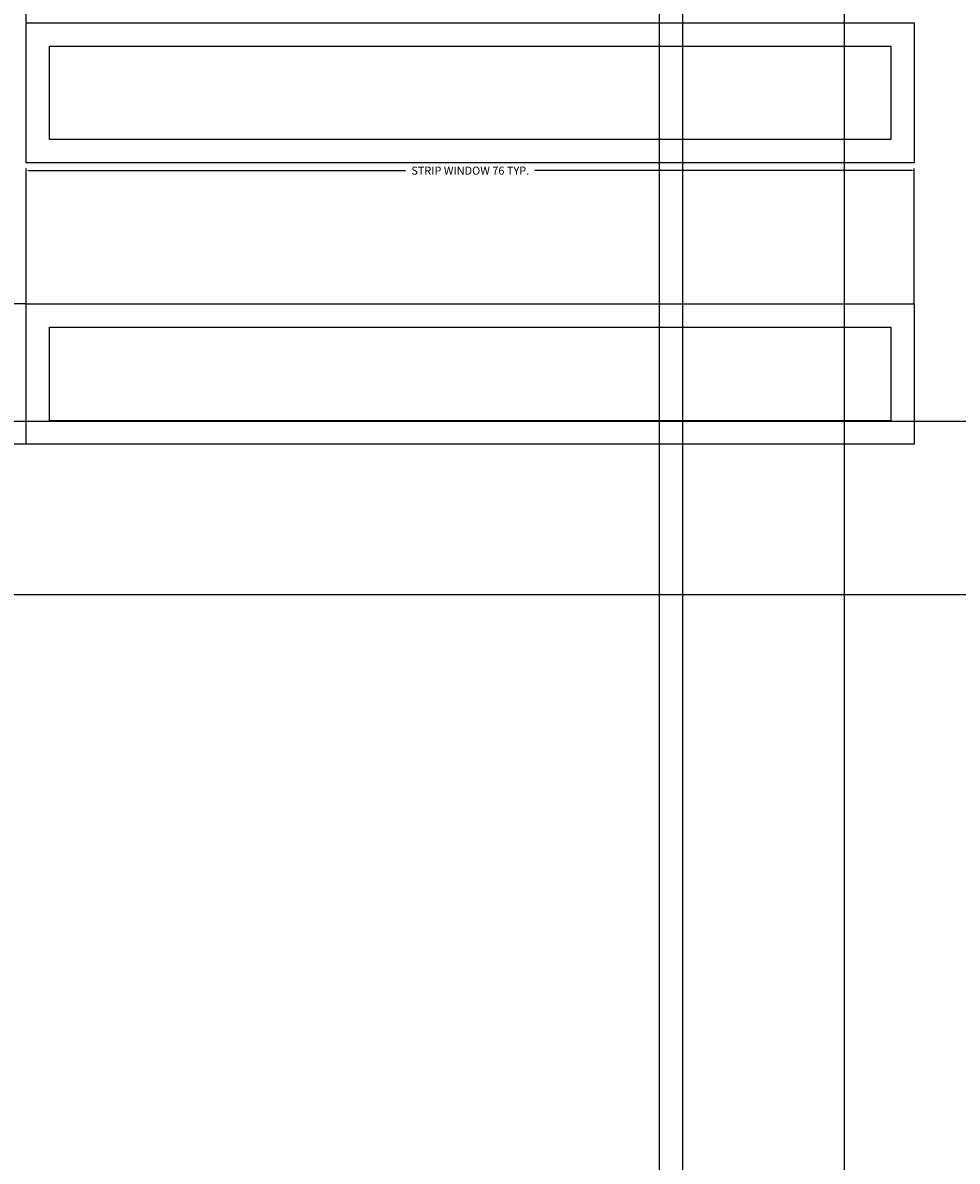
# Model space of a CAD drawing. Units: inches. Extents: x -139 to 346, y 72 to 413.
# Tile 15 of 18: x 175 to 256, y 242 to 340. Entities that reach past the tile are written whole.
import ezdxf

# ---------------------------------------------------------------- set-up
doc = ezdxf.new("R2010")
doc.units = ezdxf.units.IN
doc.header["$MEASUREMENT"] = 0
doc.layers.add('A-ANNO-DIMS', color=2, linetype='Continuous', lineweight=18)
doc.layers.add('A-GLAZ', color=4, linetype='Continuous', lineweight=25)
doc.styles.get("Standard").update_dxf_attribs({"font": 'arial.ttf'})
doc.dimstyles.get("Standard").update_dxf_attribs({"dimtxt": 0.6875, "dimasz": 0.18, "dimexe": 0.18, "dimexo": 0.0625, "dimgap": 0.09, "dimtad": 0, "dimtih": 1, "dimtoh": 1, "dimdec": 4, "dimzin": 0, "dimdsep": 46, "dimlunit": 4, "dimtxsty": 'Standard', "dimcen": 0.09, "dimadec": 0, "dimazin": 0, "dimtfac": 1, "dimtdec": 4, "dimtofl": 0, "dimtmove": 0, "dimatfit": 3, "dimfxl": 1, "dimtolj": 1, "dimtzin": 0, "dimarcsym": 0})

# ---------------------------------------------------------------- blocks, each defined once
blk = doc.blocks.new('WIN-STRIP')
for points in [[(0, 12.015), (76.156, 12.015), (76.156, 0), (0, 0)], [(2, 10.015), (74.156, 10.015), (74.156, 2), (2, 2)]]:
    blk.add_lwpolyline(points, close=True)
blk = doc.blocks.new('*D3')
at = {"layer": 'A-ANNO-DIMS', "color": 0, "lineweight": -2, "transparency": 16777216}
for p, q in [((175.668, 316.018), (175.668, 327.559)), ((175.848, 327.379), (208.196, 327.379)), ((251.644, 327.379), (219.295, 327.379)), ((251.824, 316.018), (251.824, 327.559))]:
    blk.add_line(p, q, dxfattribs=at)
at = {"layer": 'A-ANNO-DIMS', "color": 0, "transparency": 16777216}
for points in [[(175.848, 327.409), (175.848, 327.349), (175.668, 327.379)], [(251.644, 327.409), (251.644, 327.349), (251.824, 327.379)]]:
    blk.add_solid(points, dxfattribs=at)
at = {"layer": 'Defpoints', "color": 0, "transparency": 16777216}
for p in [(251.824, 327.379), (175.668, 315.955), (251.824, 315.955)]:
    blk.add_point(p, dxfattribs=at)
at = {"layer": 'A-ANNO-DIMS', "color": 0, "transparency": 16777216, "insert": (213.746, 327.379), "char_height": 0.6875, "attachment_point": 5}
blk.add_mtext('\\A1;STRIP WINDOW 76 TYP.', dxfattribs=at)
blk = doc.blocks.new('*D4')
at = {"layer": 'A-ANNO-DIMS', "color": 0, "lineweight": -2, "transparency": 16777216}
for p, q in [((175.605, 315.955), (164.064, 315.955)), ((164.244, 315.775), (164.244, 310.383)), ((164.244, 304.12), (164.244, 309.512)), ((175.605, 303.94), (164.064, 303.94))]:
    blk.add_line(p, q, dxfattribs=at)
at = {"layer": 'A-ANNO-DIMS', "color": 0, "transparency": 16777216}
for points in [[(164.214, 315.775), (164.274, 315.775), (164.244, 315.955)], [(164.214, 304.12), (164.274, 304.12), (164.244, 303.94)]]:
    blk.add_solid(points, dxfattribs=at)
at = {"layer": 'Defpoints', "color": 0, "transparency": 16777216}
for p in [(164.244, 315.955), (175.668, 315.955), (175.668, 303.94)]:
    blk.add_point(p, dxfattribs=at)
at = {"layer": 'A-ANNO-DIMS', "color": 0, "transparency": 16777216, "insert": (164.244, 309.948), "char_height": 0.6875, "attachment_point": 5}
blk.add_mtext('\\A1;12 TYP.', dxfattribs=at)
blk = doc.blocks.new('*D27')
at = {"layer": 'A-ANNO-DIMS', "color": 0, "lineweight": -2, "transparency": 16777216}
for p, q in [((112.651, 291.123), (112.651, 412.455)), ((112.831, 412.275), (142.911, 412.275)), ((175.488, 412.275), (145.407, 412.275)), ((175.668, 340.117), (175.668, 412.455))]:
    blk.add_line(p, q, dxfattribs=at)
at = {"layer": 'A-ANNO-DIMS', "color": 0, "transparency": 16777216}
for points in [[(112.831, 412.305), (112.831, 412.245), (112.651, 412.275)], [(175.488, 412.305), (175.488, 412.245), (175.668, 412.275)]]:
    blk.add_solid(points, dxfattribs=at)
at = {"layer": 'Defpoints', "color": 0, "transparency": 16777216}
for p in [(175.668, 412.275), (175.668, 340.055), (112.651, 291.06)]:
    blk.add_point(p, dxfattribs=at)
at = {"layer": 'A-ANNO-DIMS', "color": 0, "transparency": 16777216, "insert": (144.159, 412.275), "char_height": 0.6875, "attachment_point": 5}
blk.add_mtext('\\A1;63.02', dxfattribs=at)
blk = doc.blocks.new('*D80')
at = {"layer": 'A-ANNO-DIMS', "color": 0, "lineweight": -2, "transparency": 16777216}
for p, q in [((229.972, 205.587), (229.972, 412.455)), ((230.152, 412.275), (230.654, 412.275)), ((231.792, 412.275), (231.29, 412.275)), ((231.972, 203.587), (231.972, 412.455))]:
    blk.add_line(p, q, dxfattribs=at)
at = {"layer": 'A-ANNO-DIMS', "color": 0, "transparency": 16777216}
for points in [[(230.152, 412.305), (230.152, 412.245), (229.972, 412.275)], [(231.792, 412.305), (231.792, 412.245), (231.972, 412.275)]]:
    blk.add_solid(points, dxfattribs=at)
at = {"layer": 'Defpoints', "color": 0, "transparency": 16777216}
for p in [(231.972, 412.275), (229.972, 205.524), (231.972, 203.524)]:
    blk.add_point(p, dxfattribs=at)
at = {"layer": 'A-ANNO-DIMS', "color": 0, "transparency": 16777216, "insert": (230.972, 412.275), "char_height": 0.6875, "attachment_point": 5}
blk.add_mtext('\\A1;2', dxfattribs=at)
blk = doc.blocks.new('*D81')
at = {"layer": 'A-ANNO-DIMS', "color": 0, "lineweight": -2, "transparency": 16777216}
for p, q in [((231.972, 203.587), (231.972, 412.455)), ((232.152, 412.275), (237.421, 412.275)), ((245.66, 412.275), (240.391, 412.275)), ((245.84, 184.668), (245.84, 412.455))]:
    blk.add_line(p, q, dxfattribs=at)
at = {"layer": 'A-ANNO-DIMS', "color": 0, "transparency": 16777216}
for points in [[(232.152, 412.305), (232.152, 412.245), (231.972, 412.275)], [(245.66, 412.305), (245.66, 412.245), (245.84, 412.275)]]:
    blk.add_solid(points, dxfattribs=at)
at = {"layer": 'Defpoints', "color": 0, "transparency": 16777216}
for p in [(245.84, 412.275), (231.972, 203.524), (245.84, 184.606)]:
    blk.add_point(p, dxfattribs=at)
at = {"layer": 'A-ANNO-DIMS', "color": 0, "transparency": 16777216, "insert": (238.906, 412.275), "char_height": 0.6875, "attachment_point": 5}
blk.add_mtext('\\A1;13.868', dxfattribs=at)
blk = doc.blocks.new('*D82')
at = {"layer": 'A-ANNO-DIMS', "color": 0, "lineweight": -2, "transparency": 16777216}
for p, q in [((245.84, 184.668), (245.84, 412.455)), ((246.02, 412.275), (253.85, 412.275)), ((264.642, 412.275), (256.812, 412.275)), ((264.822, 184.668), (264.822, 412.455))]:
    blk.add_line(p, q, dxfattribs=at)
at = {"layer": 'A-ANNO-DIMS', "color": 0, "transparency": 16777216}
for points in [[(246.02, 412.305), (246.02, 412.245), (245.84, 412.275)], [(264.642, 412.305), (264.642, 412.245), (264.822, 412.275)]]:
    blk.add_solid(points, dxfattribs=at)
at = {"layer": 'Defpoints', "color": 0, "transparency": 16777216}
for p in [(264.822, 412.275), (245.84, 184.606), (264.822, 184.606)]:
    blk.add_point(p, dxfattribs=at)
at = {"layer": 'A-ANNO-DIMS', "color": 0, "transparency": 16777216, "insert": (255.331, 412.275), "char_height": 0.6875, "attachment_point": 5}
blk.add_mtext('\\A1;18.982', dxfattribs=at)
blk = doc.blocks.new('*D101')
at = {"layer": 'A-ANNO-DIMS', "color": 0, "lineweight": -2, "transparency": 16777216}
for p, q in [((110.387, 305.921), (344.386, 305.921)), ((344.206, 305.741), (344.206, 298.931)), ((344.206, 291.24), (344.206, 298.049)), ((112.713, 291.06), (344.386, 291.06))]:
    blk.add_line(p, q, dxfattribs=at)
at = {"layer": 'A-ANNO-DIMS', "color": 0, "transparency": 16777216}
for points in [[(344.176, 305.741), (344.236, 305.741), (344.206, 305.921)], [(344.176, 291.24), (344.236, 291.24), (344.206, 291.06)]]:
    blk.add_solid(points, dxfattribs=at)
at = {"layer": 'Defpoints', "color": 0, "transparency": 16777216}
for p in [(110.324, 305.921), (344.206, 305.921), (112.651, 291.06)]:
    blk.add_point(p, dxfattribs=at)
at = {"layer": 'A-ANNO-DIMS', "color": 0, "transparency": 16777216, "insert": (344.206, 298.49), "char_height": 0.6875, "attachment_point": 5}
blk.add_mtext('\\A1;14.86', dxfattribs=at)

msp = doc.modelspace()

# ---------------------------------------------------------------- block references
at = {"layer": 'A-GLAZ'}
for p in [(175.668, 328.04), (175.668, 303.9404)]:
    msp.add_blockref('WIN-STRIP', p, dxfattribs=at)

# ---------------------------------------------------------------- dimensions: what is measured, and where the dimension line sits
at = {"layer": 'A-ANNO-DIMS'}
for base, p1, p2, override, picture, middle in [((175.6676, 412.2748), (112.6506, 291.0604), (175.6676, 340.0548), {"dimdec": 2, "dimlfac": 1, "dimrnd": 0, "dimzin": 0, "dimdsep": 46, "dimlunit": 2}, '*D27', (144.1591, 412.2748)), ((231.972, 412.2748), (229.972, 205.5243), (231.972, 203.5243), {"dimdec": 0, "dimlfac": 1, "dimrnd": 0, "dimzin": 0, "dimdsep": 46, "dimlunit": 2}, '*D80', (230.972, 412.2748)), ((245.8399, 412.2748), (231.972, 203.5243), (245.8399, 184.6055), {"dimdec": 3, "dimlfac": 1, "dimrnd": 0, "dimzin": 0, "dimdsep": 46, "dimlunit": 2}, '*D81', (238.906, 412.2748)), ((264.8219, 412.2748), (245.8399, 184.6055), (264.8219, 184.6055), {"dimdec": 3, "dimlfac": 1, "dimrnd": 0, "dimzin": 0, "dimdsep": 46, "dimlunit": 2}, '*D82', (255.3309, 412.2748))]:
    dim = msp.add_linear_dim(base=base, p1=p1, p2=p2, dimstyle='Standard', override=override, dxfattribs=at)
    dim.commit()
    dim.dimension.update_dxf_attribs({"geometry": picture, "text_midpoint": middle})
dim = msp.add_linear_dim(base=(251.8235, 327.3786), p1=(175.6676, 315.9552), p2=(251.8235, 315.9552), text='STRIP WINDOW <> TYP.', dimstyle='Standard', override={"dimdec": 0, "dimlfac": 1, "dimrnd": 0, "dimzin": 0, "dimdsep": 46, "dimlunit": 2}, dxfattribs=at)
dim.commit()
dim.dimension.update_dxf_attribs({"geometry": '*D3', "text_midpoint": (213.7455, 327.3786)})
dim = msp.add_linear_dim(base=(164.2442, 315.9552), p1=(175.6676, 303.9402), p2=(175.6676, 315.9552), angle=90, text='<> TYP.', dimstyle='Standard', override={"dimdec": 0, "dimlfac": 1, "dimrnd": 0, "dimzin": 0, "dimdsep": 46, "dimlunit": 2}, dxfattribs=at)
dim.commit()
dim.dimension.update_dxf_attribs({"geometry": '*D4', "text_midpoint": (164.2442, 309.9477)})
dim = msp.add_linear_dim(base=(344.2055, 305.9205), p1=(112.6506, 291.0604), p2=(110.3243, 305.9205), angle=90, dimstyle='Standard', override={"dimdec": 2, "dimlfac": 1, "dimrnd": 0, "dimzin": 0, "dimdsep": 46, "dimlunit": 2}, dxfattribs=at)
dim.commit()
dim.dimension.update_dxf_attribs({"geometry": '*D101', "text_midpoint": (344.2055, 298.4905)})

doc.saveas('drawing.dxf')
